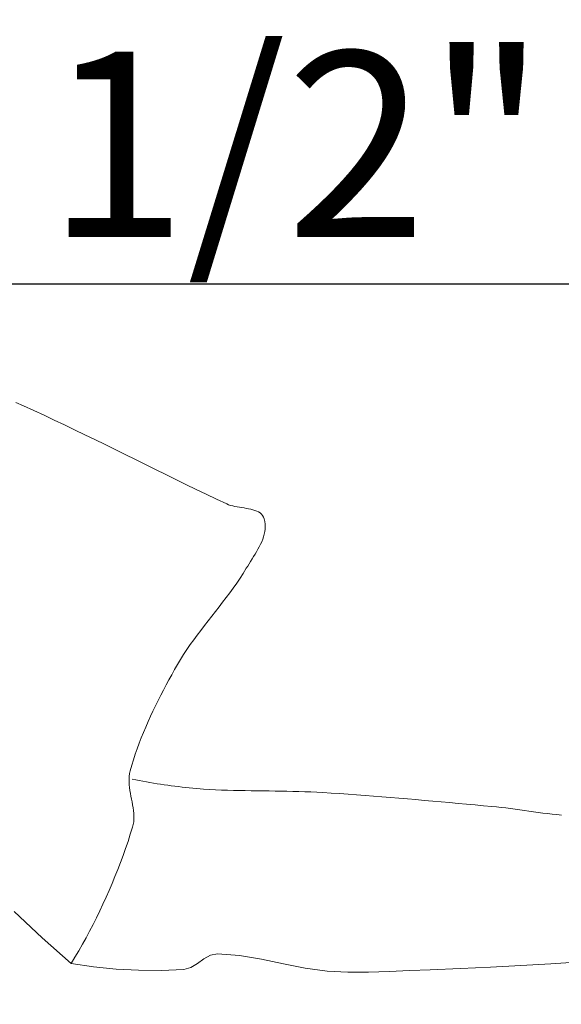
# Model space of a CAD drawing. Units: inches. Extents: x 2656 to 9931, y 1941 to 3068.
# Tile 18 of 46: x 2914 to 2932, y 2466 to 2498. Entities that reach past the tile are written whole.
import ezdxf

# ---------------------------------------------------------------- set-up
doc = ezdxf.new("R2010")
doc.units = ezdxf.units.IN
doc.layers.add('A-ANNO-DIMS', color=2, linetype='Continuous', lineweight=18)
doc.layers.add('A-FURN', color=8, linetype='Continuous', lineweight=13)
doc.styles.get("Standard").update_dxf_attribs({"font": 'arial.ttf'})
doc.dimstyles.new('ISO-25', dxfattribs={"dimtxt": 6, "dimasz": 2.5, "dimexe": 1.25, "dimexo": 0.625, "dimtad": 1, "dimdec": 0, "dimlunit": 3, "dimtxsty": 'Standard', "dimcen": 2.5, "dimadec": 0, "dimazin": 0, "dimtfac": 1, "dimtdec": 0, "dimtmove": 0, "dimatfit": 3, "dimfxl": 1, "dimarcsym": 0})

# ---------------------------------------------------------------- blocks, each defined once
blk = doc.blocks.new('BED-DOUBLE')
for p, q in [((36.853, 18.28), (36.603, 18.391)), ((37.185, 18.128), (36.853, 18.28)), ((37.515, 17.974), (37.185, 18.128)), ((37.846, 17.819), (37.515, 17.974)), ((38.175, 17.662), (37.846, 17.819)), ((38.504, 17.505), (38.175, 17.662)), ((38.832, 17.346), (38.504, 17.505)), ((39.16, 17.186), (38.832, 17.346)), ((39.488, 17.026), (39.16, 17.186)), ((39.816, 16.865), (39.488, 17.026)), ((40.143, 16.704), (39.816, 16.865)), ((40.47, 16.542), (40.143, 16.704)), ((40.797, 16.381), (40.47, 16.542)), ((41.125, 16.22), (40.797, 16.381)), ((41.452, 16.059), (41.125, 16.22)), ((41.78, 15.898), (41.452, 16.059)), ((42.107, 15.738), (41.78, 15.898)), ((42.436, 15.579), (42.107, 15.738)), ((42.764, 15.421), (42.436, 15.579)), ((43.094, 15.263), (42.764, 15.421)), ((43.424, 15.108), (43.094, 15.263)), ((43.485, 15.082), (43.424, 15.108)), ((43.55, 15.06), (43.485, 15.082)), ((43.618, 15.042), (43.55, 15.06)), ((43.689, 15.026), (43.618, 15.042)), ((43.762, 15.012), (43.689, 15.026)), ((43.836, 15), (43.762, 15.012)), ((43.91, 14.988), (43.836, 15)), ((43.985, 14.977), (43.91, 14.988)), ((44.059, 14.965), (43.985, 14.977)), ((44.131, 14.952), (44.059, 14.965)), ((44.201, 14.937), (44.131, 14.952)), ((44.269, 14.92), (44.201, 14.937)), ((44.333, 14.899), (44.269, 14.92)), ((44.394, 14.876), (44.333, 14.899)), ((44.45, 14.848), (44.394, 14.876)), ((44.501, 14.815), (44.45, 14.848)), ((44.545, 14.776), (44.501, 14.815)), ((44.584, 14.732), (44.545, 14.776)), ((44.615, 14.68), (44.584, 14.732)), ((44.638, 14.622), (44.615, 14.68)), ((44.658, 14.541), (44.638, 14.622)), ((44.67, 14.459), (44.658, 14.541)), ((44.669, 14.295), (44.673, 14.377)), ((44.673, 14.377), (44.67, 14.459)), ((44.588, 13.967), (44.617, 14.049)), ((44.617, 14.049), (44.64, 14.131)), ((44.64, 14.131), (44.658, 14.213)), ((44.658, 14.213), (44.669, 14.295)), ((44.435, 13.643), (44.478, 13.723)), ((44.478, 13.723), (44.519, 13.804)), ((44.519, 13.804), (44.556, 13.885)), ((44.556, 13.885), (44.588, 13.967)), ((44.246, 13.328), (44.294, 13.405)), ((44.294, 13.405), (44.342, 13.484)), ((44.342, 13.484), (44.389, 13.563)), ((44.389, 13.563), (44.435, 13.643)), ((44.058, 13.027), (44.103, 13.101)), ((44.103, 13.101), (44.149, 13.175)), ((44.149, 13.175), (44.197, 13.251)), ((44.197, 13.251), (44.246, 13.328)), ((43.854, 12.704), (43.958, 12.864)), ((43.958, 12.864), (44.058, 13.027)), ((43.637, 12.389), (43.747, 12.546)), ((43.747, 12.546), (43.854, 12.704)), ((43.409, 12.081), (43.524, 12.235)), ((43.524, 12.235), (43.637, 12.389)), ((43.175, 11.777), (43.293, 11.929)), ((43.293, 11.929), (43.409, 12.081)), ((42.82, 11.325), (42.938, 11.476)), ((42.938, 11.476), (43.057, 11.626)), ((43.057, 11.626), (43.175, 11.777)), ((42.585, 11.021), (42.702, 11.173)), ((42.702, 11.173), (42.82, 11.325)), ((42.356, 10.714), (42.469, 10.869)), ((42.469, 10.869), (42.585, 11.021)), ((42.136, 10.401), (42.245, 10.559)), ((42.245, 10.559), (42.356, 10.714)), ((41.93, 10.08), (42.031, 10.242)), ((42.031, 10.242), (42.136, 10.401)), ((41.739, 9.752), (41.832, 9.915)), ((41.832, 9.915), (41.93, 10.08)), ((41.555, 9.422), (41.647, 9.587)), ((41.647, 9.587), (41.739, 9.752)), ((41.377, 9.089), (41.465, 9.256)), ((41.465, 9.256), (41.555, 9.422)), ((41.204, 8.753), (41.289, 8.921)), ((41.289, 8.921), (41.377, 9.089)), ((41.12, 8.583), (41.204, 8.753)), ((40.958, 8.242), (41.038, 8.413)), ((41.038, 8.413), (41.12, 8.583)), ((40.805, 7.896), (40.88, 8.069)), ((40.88, 8.069), (40.958, 8.242)), ((40.661, 7.547), (40.732, 7.722)), ((40.732, 7.722), (40.805, 7.896)), ((40.529, 7.195), (40.594, 7.371)), ((40.594, 7.371), (40.661, 7.547)), ((40.408, 6.838), (40.467, 7.017)), ((40.467, 7.017), (40.529, 7.195)), ((40.353, 6.658), (40.408, 6.838)), ((40.269, 6.3), (40.281, 6.389)), ((40.281, 6.389), (40.301, 6.477)), ((40.301, 6.477), (40.353, 6.658)), ((40.264, 6.21), (40.269, 6.3)), ((40.264, 6.119), (40.264, 6.21)), ((40.27, 6.028), (40.264, 6.119)), ((40.368, 6.212), (40.482, 6.189)), ((40.482, 6.189), (40.596, 6.166)), ((40.596, 6.166), (40.711, 6.144)), ((40.711, 6.144), (40.826, 6.123)), ((40.826, 6.123), (40.941, 6.103)), ((40.941, 6.103), (41.056, 6.083)), ((41.056, 6.083), (41.171, 6.064)), ((41.171, 6.064), (41.286, 6.046)), ((40.281, 5.936), (40.27, 6.028)), ((40.294, 5.844), (40.281, 5.936)), ((40.31, 5.751), (40.294, 5.844)), ((40.328, 5.659), (40.31, 5.751)), ((41.286, 6.046), (41.402, 6.029)), ((41.402, 6.029), (41.517, 6.012)), ((41.517, 6.012), (41.633, 5.997)), ((41.633, 5.997), (41.749, 5.982)), ((41.749, 5.982), (41.864, 5.968)), ((41.864, 5.968), (41.98, 5.954)), ((41.98, 5.954), (42.096, 5.942)), ((42.096, 5.942), (42.213, 5.93)), ((42.213, 5.93), (42.329, 5.919)), ((42.329, 5.919), (42.445, 5.909)), ((42.445, 5.909), (42.561, 5.899)), ((42.561, 5.899), (42.677, 5.891)), ((42.677, 5.891), (42.87, 5.878)), ((42.87, 5.878), (43.062, 5.868)), ((43.062, 5.868), (43.254, 5.859)), ((43.254, 5.859), (43.447, 5.852)), ((43.447, 5.852), (43.639, 5.846)), ((43.639, 5.846), (43.832, 5.841)), ((43.832, 5.841), (44.024, 5.838)), ((44.024, 5.838), (44.217, 5.834)), ((44.217, 5.834), (44.41, 5.832)), ((44.41, 5.832), (44.602, 5.83)), ((44.602, 5.83), (44.795, 5.828)), ((44.795, 5.828), (44.988, 5.825)), ((44.988, 5.825), (45.18, 5.823)), ((45.18, 5.823), (45.373, 5.82)), ((45.373, 5.82), (45.566, 5.816)), ((45.566, 5.816), (45.758, 5.811)), ((45.758, 5.811), (45.951, 5.805)), ((45.951, 5.805), (46.143, 5.798)), ((46.143, 5.798), (46.336, 5.789)), ((46.336, 5.789), (46.528, 5.778)), ((46.528, 5.778), (46.802, 5.761)), ((46.802, 5.761), (47.076, 5.743)), ((47.076, 5.743), (47.35, 5.724)), ((40.347, 5.566), (40.328, 5.659)), ((40.365, 5.473), (40.347, 5.566)), ((40.382, 5.381), (40.365, 5.473)), ((47.35, 5.724), (47.624, 5.705)), ((47.624, 5.705), (47.898, 5.684)), ((47.898, 5.684), (48.172, 5.663)), ((48.172, 5.663), (48.445, 5.641)), ((48.445, 5.641), (48.719, 5.619)), ((48.719, 5.619), (48.993, 5.596)), ((48.993, 5.596), (49.266, 5.573)), ((49.266, 5.573), (49.54, 5.549)), ((49.54, 5.549), (49.813, 5.525)), ((49.813, 5.525), (50.087, 5.5)), ((50.087, 5.5), (50.36, 5.476)), ((50.36, 5.476), (50.634, 5.451)), ((50.634, 5.451), (50.907, 5.426)), ((50.907, 5.426), (51.181, 5.402)), ((40.398, 5.288), (40.382, 5.381)), ((40.411, 5.196), (40.398, 5.288)), ((40.42, 5.105), (40.411, 5.196)), ((40.424, 5.014), (40.42, 5.105)), ((51.181, 5.402), (51.454, 5.377)), ((51.454, 5.377), (51.728, 5.352)), ((51.728, 5.352), (52.002, 5.328)), ((52.002, 5.328), (52.151, 5.313)), ((52.151, 5.313), (52.301, 5.297)), ((52.301, 5.297), (52.451, 5.279)), ((52.451, 5.279), (52.601, 5.26)), ((52.601, 5.26), (52.75, 5.239)), ((52.75, 5.239), (52.9, 5.218)), ((52.9, 5.218), (53.05, 5.197)), ((53.05, 5.197), (53.199, 5.176)), ((53.199, 5.176), (53.349, 5.155)), ((53.349, 5.155), (53.498, 5.134)), ((53.498, 5.134), (53.648, 5.114)), ((53.648, 5.114), (53.798, 5.095)), ((53.798, 5.095), (53.947, 5.078)), ((40.402, 4.746), (40.416, 4.834)), ((40.416, 4.834), (40.424, 4.924)), ((40.424, 4.924), (40.424, 5.014)), ((53.947, 5.078), (54.097, 5.062)), ((54.097, 5.062), (54.247, 5.049)), ((40.307, 4.427), (40.38, 4.658)), ((40.38, 4.658), (40.402, 4.746)), ((40.154, 3.968), (40.232, 4.197)), ((40.232, 4.197), (40.307, 4.427)), ((40.072, 3.739), (40.154, 3.968)), ((39.901, 3.285), (39.988, 3.512)), ((39.988, 3.512), (40.072, 3.739)), ((39.811, 3.06), (39.901, 3.285)), ((39.718, 2.835), (39.811, 3.06)), ((39.524, 2.39), (39.623, 2.612)), ((39.623, 2.612), (39.718, 2.835)), ((39.423, 2.169), (39.524, 2.39)), ((36.55, 1.936), (37.459, 1.078)), ((39.213, 1.731), (39.319, 1.949)), ((39.319, 1.949), (39.423, 2.169)), ((39.103, 1.515), (39.213, 1.731)), ((38.876, 1.085), (38.991, 1.299)), ((38.991, 1.299), (39.103, 1.515)), ((37.459, 1.078), (38.392, 0.247)), ((38.759, 0.873), (38.876, 1.085)), ((38.517, 0.454), (38.639, 0.663)), ((38.639, 0.663), (38.759, 0.873)), ((38.392, 0.247), (38.517, 0.454)), ((42.478, 0.252), (42.684, 0.399)), ((42.684, 0.399), (42.897, 0.52)), ((42.897, 0.52), (43.125, 0.568)), ((43.125, 0.568), (43.84, 0.512)), ((43.84, 0.512), (44.549, 0.388)), ((44.549, 0.388), (45.256, 0.236)), ((38.392, 0.247), (39.115, 0.14)), ((39.115, 0.14), (39.844, 0.068)), ((39.844, 0.068), (40.575, 0.031)), ((40.575, 0.031), (41.307, 0.028)), ((41.307, 0.028), (42.038, 0.06)), ((42.038, 0.06), (42.266, 0.124)), ((42.266, 0.124), (42.478, 0.252)), ((45.256, 0.236), (45.964, 0.094)), ((45.964, 0.094), (46.677, 0.002)), ((46.677, 0.002), (47.342, -0.03)), ((48.675, -0.01), (49.342, 0.02)), ((49.342, 0.02), (50.009, 0.048)), ((50.009, 0.048), (50.984, 0.088)), ((50.984, 0.088), (51.958, 0.135)), ((51.958, 0.135), (52.933, 0.187)), ((52.933, 0.187), (53.907, 0.244)), ((53.907, 0.244), (54.881, 0.304)), ((47.342, -0.03), (48.009, -0.03)), ((48.009, -0.03), (48.675, -0.01))]:
    blk.add_line(p, q)
blk = doc.blocks.new('*D31')
at = {"layer": 'A-ANNO-DIMS', "color": 0, "lineweight": -2, "transparency": 16777216}
for p, q in [((2753.358, 2502.145), (2753.358, 2488.227)), ((2841.982, 2502.145), (2841.982, 2488.227)), ((2755.858, 2489.477), (2839.482, 2489.477)), ((2841.982, 2489.477), (2952.348, 2489.477))]:
    blk.add_line(p, q, dxfattribs=at)
at = {"layer": 'A-ANNO-DIMS', "color": 0, "transparency": 16777216}
for points in [[(2755.858, 2489.893), (2755.858, 2489.06), (2753.358, 2489.477)], [(2839.482, 2489.893), (2839.482, 2489.06), (2841.982, 2489.477)]]:
    blk.add_solid(points, dxfattribs=at)
at = {"layer": 'Defpoints', "color": 0, "transparency": 16777216}
for p in [(2753.358, 2502.77), (2841.982, 2502.77), (2841.982, 2489.477)]:
    blk.add_point(p, dxfattribs=at)
at = {"layer": 'A-ANNO-DIMS', "color": 0, "transparency": 16777216, "insert": (2898.415, 2493.206), "char_height": 6, "attachment_point": 5}
blk.add_mtext('DOUBLE BED 7\'-4 1/2" TYP.', dxfattribs=at)
blk = doc.blocks.new('*D102')
at = {"layer": 'A-ANNO-DIMS', "color": 0, "lineweight": -2, "transparency": 16777216}
for p, q in [((2998.157, 2604.975), (2998.157, 2009.273)), ((2872.157, 2564.712), (2872.157, 2009.273)), ((2874.657, 2010.523), (2995.657, 2010.523))]:
    blk.add_line(p, q, dxfattribs=at)
at = {"layer": 'A-ANNO-DIMS', "color": 0, "transparency": 16777216}
for points in [[(2874.657, 2010.939), (2874.657, 2010.106), (2872.157, 2010.523)], [(2995.657, 2010.939), (2995.657, 2010.106), (2998.157, 2010.523)]]:
    blk.add_solid(points, dxfattribs=at)
at = {"layer": 'Defpoints', "color": 0, "transparency": 16777216}
for p in [(2998.157, 2605.6), (2872.157, 2565.337), (2998.157, 2010.523)]:
    blk.add_point(p, dxfattribs=at)
at = {"layer": 'A-ANNO-DIMS', "color": 0, "transparency": 16777216, "insert": (2935.157, 2014.211), "char_height": 6, "attachment_point": 5}
blk.add_mtext('10\'-6"', dxfattribs=at)
blk = doc.blocks.new('*D130')
at = {"layer": 'A-ANNO-DIMS', "color": 0, "lineweight": -2, "transparency": 16777216}
for p, q in [((2877.282, 2538.52), (3061.007, 2538.52)), ((3059.757, 2536.02), (3059.757, 2525.316)), ((2902.165, 2522.816), (3061.007, 2522.816)), ((3059.757, 2522.816), (3059.757, 2489.7))]:
    blk.add_line(p, q, dxfattribs=at)
at = {"layer": 'A-ANNO-DIMS', "color": 0, "transparency": 16777216}
for points in [[(3059.341, 2536.02), (3060.174, 2536.02), (3059.757, 2538.52)], [(3059.341, 2525.316), (3060.174, 2525.316), (3059.757, 2522.816)]]:
    blk.add_solid(points, dxfattribs=at)
at = {"layer": 'Defpoints', "color": 0, "transparency": 16777216}
for p in [(2876.657, 2538.52), (2901.54, 2522.816), (3059.757, 2522.816)]:
    blk.add_point(p, dxfattribs=at)
at = {"layer": 'A-ANNO-DIMS', "color": 0, "transparency": 16777216, "insert": (3056.028, 2505.008), "char_height": 6, "attachment_point": 5, "rotation": 90}
blk.add_mtext('1\'-3 1/2"', dxfattribs=at)

msp = doc.modelspace()

# ---------------------------------------------------------------- block references
at = {"layer": 'A-FURN'}
msp.add_blockref('BED-DOUBLE', (2877.353, 2467.251), dxfattribs=at)

# ---------------------------------------------------------------- dimensions: what is measured, and where the dimension line sits
at = {"layer": 'A-ANNO-DIMS'}
dim = msp.add_linear_dim(base=(2998.157, 2010.523), p1=(2872.157, 2565.337), p2=(2998.157, 2605.6), dimstyle='ISO-25', override={"dimdec": 1, "dimlfac": 1, "dimrnd": 0, "dimzin": 1, "dimdsep": 46, "dimlunit": 4, "dimfrac": 2}, dxfattribs=at)
dim.commit()
dim.dimension.update_dxf_attribs({"geometry": '*D102', "text_midpoint": (2935.157, 2014.211)})
dim = msp.add_linear_dim(base=(3059.757, 2522.816), p1=(2876.657, 2538.52), p2=(2901.54, 2522.816), angle=90, dimstyle='ISO-25', override={"dimdec": 1, "dimlfac": 1, "dimrnd": 0, "dimzin": 1, "dimdsep": 46, "dimlunit": 4, "dimfrac": 2}, dxfattribs=at)
dim.commit()
dim.dimension.update_dxf_attribs({"geometry": '*D130', "text_midpoint": (3056.028, 2505.008)})
dim = msp.add_linear_dim(base=(2841.982, 2489.477), p1=(2753.358, 2502.77), p2=(2841.982, 2502.77), text='DOUBLE BED <> TYP.', dimstyle='ISO-25', override={"dimdec": 1, "dimlfac": 1, "dimrnd": 0, "dimzin": 1, "dimdsep": 46, "dimlunit": 4, "dimfrac": 2}, dxfattribs=at)
dim.commit()
dim.dimension.update_dxf_attribs({"geometry": '*D31', "text_midpoint": (2898.415, 2493.206)})

doc.saveas('drawing.dxf')
